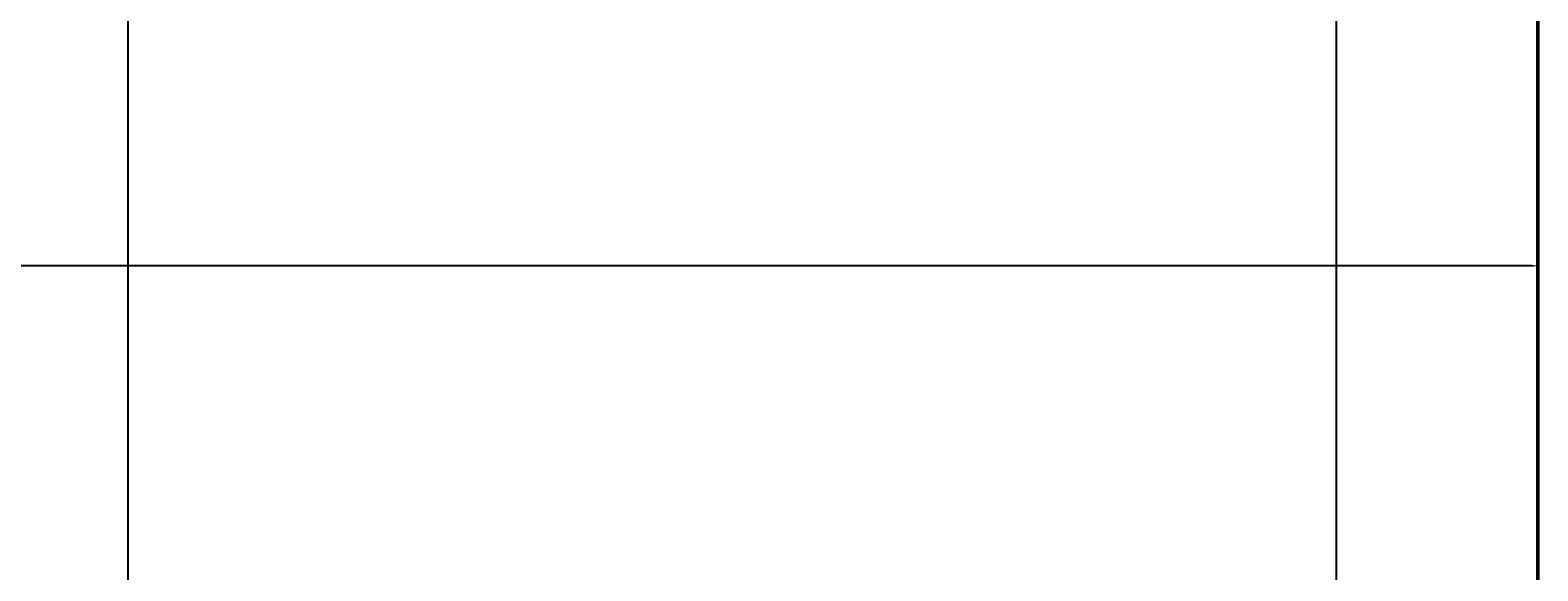
# Model space of a CAD drawing. Units: inches. Extents: x 0 to 281, y -535 to 46.
# Tile 16 of 22: x 112 to 156, y -82 to -66. Entities that reach past the tile are written whole.
import ezdxf

# ---------------------------------------------------------------- set-up
doc = ezdxf.new("R2010")
doc.units = ezdxf.units.IN
doc.header["$MEASUREMENT"] = 0
doc.layers.add('A-ANNO-DIMS', color=2, linetype='Continuous', lineweight=18)
doc.layers.add('A-WALL', color=7, linetype='Continuous', lineweight=50)
doc.styles.get("Standard").update_dxf_attribs({"font": 'arial.ttf'})
doc.dimstyles.get("Standard").update_dxf_attribs({"dimtxt": 0.18, "dimasz": 0.18, "dimexe": 0.18, "dimexo": 0.0625, "dimgap": 0.09, "dimtad": 0, "dimtih": 1, "dimtoh": 1, "dimdec": 0, "dimzin": 0, "dimdsep": 46, "dimlunit": 3, "dimtxsty": 'Standard', "dimcen": 0.09, "dimadec": 0, "dimazin": 0, "dimtfac": 1, "dimtdec": 0, "dimtofl": 0, "dimtmove": 0, "dimatfit": 3, "dimfxl": 1, "dimtolj": 1, "dimtzin": 0, "dimarcsym": 0})

# ---------------------------------------------------------------- blocks, each defined once
blk = doc.blocks.new('*D2')
at = {"layer": 'A-ANNO-DIMS', "color": 0, "lineweight": -2, "transparency": 16777216}
for p, q in [((36.459, -73.027), (36.459, -72.91)), ((36.639, -73.09), (91.56, -73.09)), ((156.279, -73.09), (101.358, -73.09)), ((156.459, -73.027), (156.459, -72.91))]:
    blk.add_line(p, q, dxfattribs=at)
at = {"layer": 'A-ANNO-DIMS', "color": 0, "transparency": 16777216}
for points in [[(36.639, -73.06), (36.639, -73.12), (36.459, -73.09)], [(156.279, -73.06), (156.279, -73.12), (156.459, -73.09)]]:
    blk.add_solid(points, dxfattribs=at)
at = {"layer": 'Defpoints', "color": 0, "transparency": 16777216}
for p in [(36.459, -73.09), (156.459, -73.09), (156.459, -73.09)]:
    blk.add_point(p, dxfattribs=at)
at = {"layer": 'A-ANNO-DIMS', "color": 0, "transparency": 16777216, "insert": (96.459, -73.09), "char_height": 6, "attachment_point": 5}
blk.add_mtext("\\A1;10'", dxfattribs=at)
blk = doc.blocks.new('*D45')
at = {"layer": 'A-ANNO-DIMS', "color": 0, "lineweight": -2, "transparency": 16777216}
for p, q in [((114.459, -263.348), (114.459, 46.219)), ((114.639, 46.039), (132.13, 46.039)), ((150.279, 46.039), (132.788, 46.039)), ((150.459, -263.348), (150.459, 46.219))]:
    blk.add_line(p, q, dxfattribs=at)
at = {"layer": 'A-ANNO-DIMS', "color": 0, "transparency": 16777216}
for points in [[(114.639, 46.069), (114.639, 46.009), (114.459, 46.039)], [(150.279, 46.069), (150.279, 46.009), (150.459, 46.039)]]:
    blk.add_solid(points, dxfattribs=at)
at = {"layer": 'Defpoints', "color": 0, "transparency": 16777216}
for p in [(150.459, 46.039), (114.459, -263.411), (150.459, -263.411)]:
    blk.add_point(p, dxfattribs=at)
at = {"layer": 'A-ANNO-DIMS', "color": 0, "transparency": 16777216, "insert": (132.459, 46.039), "char_height": 0.18, "attachment_point": 5}
blk.add_mtext('\\A1;3\'-0"', dxfattribs=at)
blk = doc.blocks.new('*D47')
at = {"layer": 'A-ANNO-DIMS', "color": 0, "lineweight": -2, "transparency": 16777216}
for p, q in [((114.459, -392.348), (114.459, 46.219)), ((114.639, 46.039), (132.13, 46.039)), ((150.279, 46.039), (132.788, 46.039)), ((150.459, -392.348), (150.459, 46.219))]:
    blk.add_line(p, q, dxfattribs=at)
at = {"layer": 'A-ANNO-DIMS', "color": 0, "transparency": 16777216}
for points in [[(114.639, 46.069), (114.639, 46.009), (114.459, 46.039)], [(150.279, 46.069), (150.279, 46.009), (150.459, 46.039)]]:
    blk.add_solid(points, dxfattribs=at)
at = {"layer": 'Defpoints', "color": 0, "transparency": 16777216}
for p in [(150.459, 46.039), (114.459, -392.411), (150.459, -392.411)]:
    blk.add_point(p, dxfattribs=at)
at = {"layer": 'A-ANNO-DIMS', "color": 0, "transparency": 16777216, "insert": (132.459, 46.039), "char_height": 0.18, "attachment_point": 5}
blk.add_mtext('\\A1;3\'-0"', dxfattribs=at)

msp = doc.modelspace()

# ---------------------------------------------------------------- linework, layer by layer
at = {"layer": 'A-WALL'}
msp.add_line((156.459, 18.589), (156.459, -131.411), dxfattribs=at)

# ---------------------------------------------------------------- dimensions: what is measured, and where the dimension line sits
at = {"layer": 'A-ANNO-DIMS'}
for base, p1, p2, override, picture, middle in [((150.459, 46.039), (114.459, -263.411), (150.459, -263.411), {"dimdec": 1, "dimlfac": 1, "dimrnd": 0, "dimzin": 1, "dimdsep": 46, "dimlunit": 4, "dimfrac": 2}, '*D45', (132.459, 46.039)), ((150.459, 46.039), (114.459, -392.411), (150.459, -392.411), {"dimdec": 1, "dimlfac": 1, "dimrnd": 0, "dimzin": 1, "dimdsep": 46, "dimlunit": 4, "dimfrac": 2}, '*D47', (132.459, 46.039)), ((156.459, -73.09), (36.459, -73.09), (156.459, -73.09), {"dimtxt": 6, "dimclrd": 0, "dimclre": 0, "dimclrt": 0}, '*D2', (96.459, -73.09))]:
    dim = msp.add_linear_dim(base=base, p1=p1, p2=p2, dimstyle='Standard', override=override, dxfattribs=at)
    dim.commit()
    dim.dimension.update_dxf_attribs({"geometry": picture, "text_midpoint": middle})

doc.saveas('drawing.dxf')
